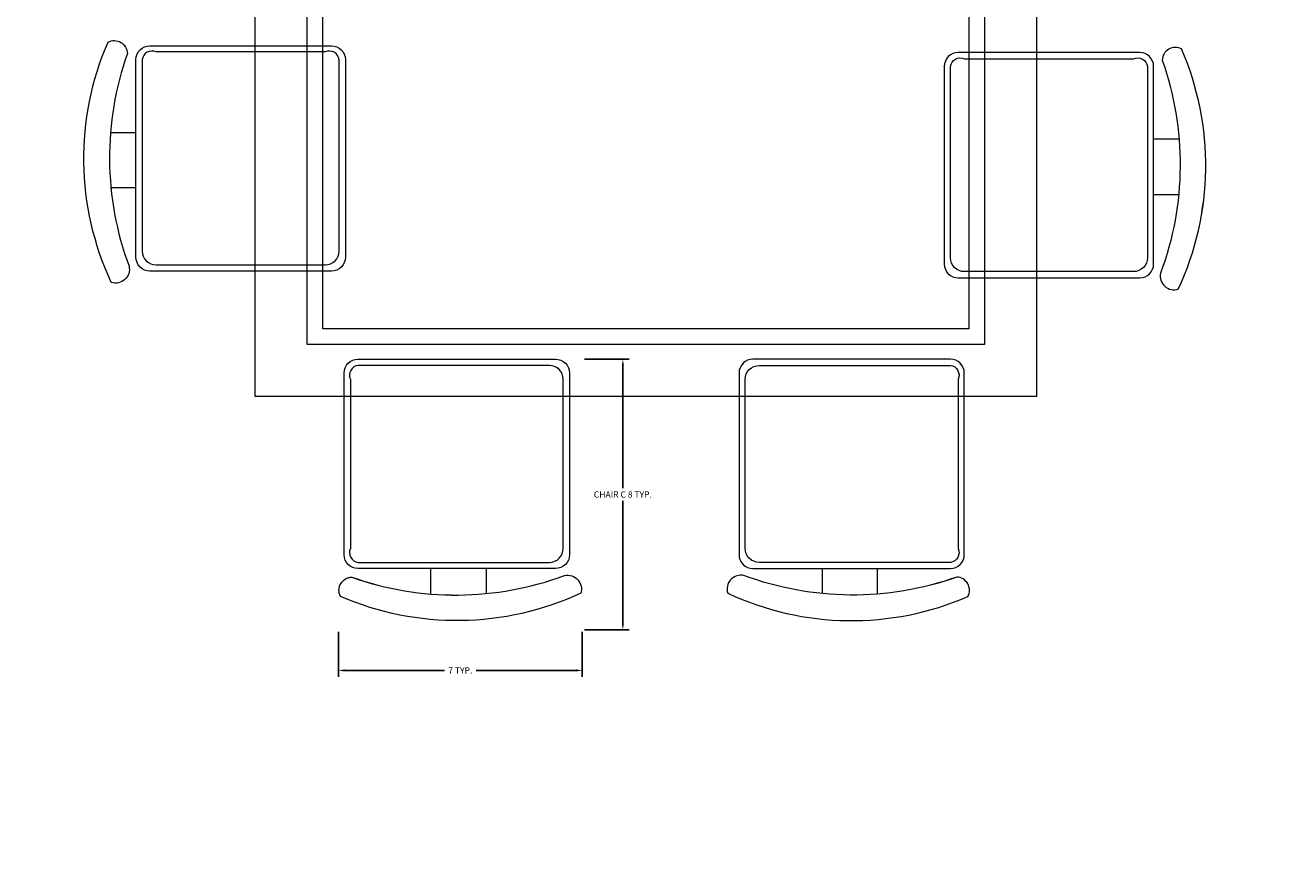
# Model space of a CAD drawing. Units: inches. Extents: x 1962 to 2771, y 1245 to 2660.
# Tile 87 of 114: x 2272 to 2308, y 2260 to 2284. Entities that reach past the tile are written whole.
import ezdxf

# ---------------------------------------------------------------- set-up
doc = ezdxf.new("R2010")
doc.units = ezdxf.units.IN
doc.layers.add('A-ANNO-DIMS', color=2, linetype='Continuous', lineweight=18)
doc.layers.add('A-FURN', color=8, linetype='Continuous', lineweight=13)
doc.styles.get("Standard").update_dxf_attribs({"font": 'arial.ttf'})
doc.dimstyles.get("Standard").update_dxf_attribs({"dimtxt": 0.18, "dimasz": 0.18, "dimexe": 0.18, "dimexo": 0.0625, "dimgap": 0.09, "dimtad": 0, "dimtih": 1, "dimtoh": 1, "dimdec": 4, "dimzin": 0, "dimdsep": 46, "dimtxsty": 'Standard', "dimcen": 0.09, "dimadec": 0, "dimazin": 0, "dimtfac": 1, "dimtdec": 4, "dimtofl": 0, "dimtmove": 0, "dimatfit": 3, "dimfxl": 1, "dimtolj": 1, "dimtzin": 0, "dimarcsym": 0})

# ---------------------------------------------------------------- blocks, each defined once
blk = doc.blocks.new('DINING-TABLE')
for points in [[(0, 13.512), (22.52, 13.512), (22.52, 0), (0, 0)], [(0, 13.512), (22.52, 13.512), (22.52, 0), (0, 0)], [(1.501, 12.011), (21.019, 12.011), (21.019, 1.502), (1.501, 1.502)], [(1.501, 12.011), (21.019, 12.011), (21.019, 1.501), (1.501, 1.501)], [(1.952, 11.561), (20.568, 11.561), (20.568, 1.952), (1.952, 1.952)], [(1.952, 11.56), (20.568, 11.56), (20.568, 1.952), (1.952, 1.952)]]:
    blk.add_lwpolyline(points, close=True)
blk = doc.blocks.new('DINING-CHAIR-C')
for points in [[(6.242, 1.501), (0.548, 1.501, -0.414214), (0.149, 1.899), (0.149, 7.135, -0.414214), (0.548, 7.534), (6.242, 7.534, -0.414214), (6.64, 7.135), (6.64, 1.899, -0.414214), (6.242, 1.501)], [(6.242, 1.501), (0.548, 1.501, -0.414214), (0.149, 1.899), (0.149, 7.135, -0.414214), (0.548, 7.533), (6.242, 7.533, -0.414214), (6.641, 7.135), (6.641, 1.899, -0.414214), (6.242, 1.501)], [(4.242, 1.501), (4.242, 0.781, 0.064759)], [(4.242, 1.501), (4.242, 0.78, 0.064759)], [(6.502, 1.301, -0.578392), (6.967, 0.79, -0.214524), (0.043, 0.697, -0.552014), (0.368, 1.255, 0.175809), (6.502, 1.301)], [(6.502, 1.301, -0.578392), (6.967, 0.79, -0.214524), (0.043, 0.697, -0.552014), (0.368, 1.254, 0.175809), (6.502, 1.301)]]:
    blk.add_lwpolyline(points, format="xyb")
for points in [[(0.55, 1.68), (6.063, 1.68, 0.414214), (6.461, 2.079), (6.461, 6.956, 0.414214), (6.063, 7.354), (0.55, 7.354, 0.512069), (0.329, 6.956), (0.329, 2.079, 0.512069)], [(0.55, 1.68), (6.063, 1.68, 0.414214), (6.461, 2.078), (6.461, 6.955, 0.414214), (6.063, 7.354), (0.55, 7.354, 0.512069), (0.329, 6.955), (0.329, 2.078, 0.512069)]]:
    blk.add_lwpolyline(points, format="xyb", close=True)
for points in [[(2.648, 0.768), (2.648, 1.501)], [(2.648, 0.767), (2.648, 1.501)]]:
    blk.add_lwpolyline(points)
blk = doc.blocks.new('*D38')
at = {"layer": 'A-ANNO-DIMS', "color": 0, "lineweight": -2, "transparency": 16777216}
for p, q in [((2288.118, 2274.618), (2289.405, 2274.618)), ((2289.225, 2274.438), (2289.225, 2270.903)), ((2289.225, 2267.001), (2289.225, 2270.537)), ((2288.118, 2266.821), (2289.405, 2266.821))]:
    blk.add_line(p, q, dxfattribs=at)
at = {"layer": 'A-ANNO-DIMS', "color": 0, "transparency": 16777216}
for points in [[(2289.195, 2274.438), (2289.255, 2274.438), (2289.225, 2274.618)], [(2289.195, 2267.001), (2289.255, 2267.001), (2289.225, 2266.821)]]:
    blk.add_solid(points, dxfattribs=at)
at = {"layer": 'Defpoints', "color": 0, "transparency": 16777216}
for p in [(2288.056, 2274.618), (2289.225, 2274.618), (2288.056, 2266.821)]:
    blk.add_point(p, dxfattribs=at)
at = {"layer": 'A-ANNO-DIMS', "color": 0, "transparency": 16777216, "insert": (2289.225, 2270.72), "char_height": 0.18, "attachment_point": 5}
blk.add_mtext('\\A1;CHAIR C 8 TYP.', dxfattribs=at)
blk = doc.blocks.new('*D39')
at = {"layer": 'A-ANNO-DIMS', "color": 0, "lineweight": -2, "transparency": 16777216}
for p, q in [((2281.028, 2266.759), (2281.028, 2265.471)), ((2288.056, 2266.759), (2288.056, 2265.471)), ((2281.208, 2265.651), (2284.084, 2265.651)), ((2287.876, 2265.651), (2284.999, 2265.651))]:
    blk.add_line(p, q, dxfattribs=at)
at = {"layer": 'A-ANNO-DIMS', "color": 0, "transparency": 16777216}
for points in [[(2281.208, 2265.681), (2281.208, 2265.621), (2281.028, 2265.651)], [(2287.876, 2265.681), (2287.876, 2265.621), (2288.056, 2265.651)]]:
    blk.add_solid(points, dxfattribs=at)
at = {"layer": 'Defpoints', "color": 0, "transparency": 16777216}
for p in [(2281.028, 2266.821), (2288.056, 2266.821), (2288.056, 2265.651)]:
    blk.add_point(p, dxfattribs=at)
at = {"layer": 'A-ANNO-DIMS', "color": 0, "transparency": 16777216, "insert": (2284.542, 2265.651), "char_height": 0.18, "attachment_point": 5}
blk.add_mtext('\\A1;7 TYP.', dxfattribs=at)
blk = doc.blocks.new('*D40')
at = {"layer": 'A-ANNO-DIMS', "color": 0, "lineweight": -2, "transparency": 16777216}
for p, q in [((2072.02, 2033.906), (2072.02, 2583.474)), ((2660.807, 2524.406), (2660.807, 2583.474)), ((2072.2, 2583.294), (2366.02, 2583.294)), ((2660.627, 2583.294), (2366.808, 2583.294))]:
    blk.add_line(p, q, dxfattribs=at)
at = {"layer": 'A-ANNO-DIMS', "color": 0, "transparency": 16777216}
for points in [[(2072.2, 2583.324), (2072.2, 2583.264), (2072.02, 2583.294)], [(2660.627, 2583.324), (2660.627, 2583.264), (2660.807, 2583.294)]]:
    blk.add_solid(points, dxfattribs=at)
at = {"layer": 'Defpoints', "color": 0, "transparency": 16777216}
for p in [(2660.807, 2583.294), (2660.807, 2524.344), (2072.02, 2033.844)]:
    blk.add_point(p, dxfattribs=at)
at = {"layer": 'A-ANNO-DIMS', "color": 0, "transparency": 16777216, "insert": (2366.414, 2583.294), "char_height": 0.18, "attachment_point": 5}
blk.add_mtext('\\A1;588.8', dxfattribs=at)

msp = doc.modelspace()

# ---------------------------------------------------------------- linework, layer by layer
at = {"layer": 'A-FURN'}
for points in [[(2274.9962, 2277.2945, -0.5783921), (2274.4852, 2276.8298, -0.2145244), (2274.3923, 2283.7537, -0.552014), (2274.9497, 2283.4284, 0.1758094), (2274.9962, 2277.2945)], [(2274.9962, 2277.2943, -0.5783921), (2274.4852, 2276.8296, -0.2145244), (2274.3923, 2283.7534, -0.552014), (2274.9497, 2283.4282, 0.1758094), (2274.9962, 2277.2943)], [(2275.1959, 2283.2492, -0.4142136), (2275.5943, 2283.6476), (2280.8302, 2283.6476, -0.4142136), (2281.2286, 2283.2492), (2281.2286, 2277.5548, -0.4142136), (2280.8302, 2277.1564), (2275.5943, 2277.1564, -0.4142136), (2275.1959, 2277.5548), (2275.1959, 2283.2492)], [(2275.1959, 2283.249, -0.4142136), (2275.5943, 2283.6474), (2280.8303, 2283.6474, -0.4142136), (2281.2286, 2283.249), (2281.2286, 2277.5545, -0.4142136), (2280.8303, 2277.1561), (2275.5943, 2277.1561, -0.4142136), (2275.1959, 2277.5545), (2275.1959, 2283.249)], [(2304.7659, 2283.2334, -0.1758092), (2304.7195, 2277.0995, 0.5783921), (2305.2304, 2276.6348, 0.2145244), (2305.3233, 2283.5587, 0.552014), (2304.7659, 2283.2334, -0.065079)], [(2304.7659, 2283.2331, -0.1758092), (2304.7195, 2277.0993, 0.5783921), (2305.2305, 2276.6346, 0.2145244), (2305.3234, 2283.5584, 0.552014), (2304.7659, 2283.2331, -0.065079)], [(2304.5197, 2283.0542, 0.4142136), (2304.1214, 2283.4526), (2298.8854, 2283.4526, 0.4142136), (2298.487, 2283.0542), (2298.487, 2277.3597, 0.4142136), (2298.8854, 2276.9614), (2304.1214, 2276.9614, 0.4142136), (2304.5197, 2277.3597), (2304.5197, 2283.0542)], [(2304.5198, 2283.054, 0.4142136), (2304.1214, 2283.4524), (2298.8854, 2283.4524, 0.4142136), (2298.487, 2283.054), (2298.487, 2277.3595, 0.4142136), (2298.8854, 2276.9611), (2304.1214, 2276.9611, 0.4142136), (2304.5198, 2277.3595), (2304.5198, 2283.054)], [(2275.1959, 2279.5549), (2274.4757, 2279.5549, 0.0647586)], [(2275.1959, 2279.5547), (2274.4757, 2279.5547, 0.0647586)], [(2304.5197, 2279.3599), (2305.2399, 2279.3599, -0.0647586)], [(2304.5198, 2279.3597), (2305.2399, 2279.3597, -0.0647586)], [(2298.6658, 2268.5856, 0.4142136), (2299.0642, 2268.984), (2299.0642, 2274.2199, 0.4142136), (2298.6658, 2274.6183), (2292.9714, 2274.6183, 0.4142136), (2292.573, 2274.2199), (2292.573, 2268.984, 0.4142136), (2292.9714, 2268.5856), (2298.6658, 2268.5856)], [(2298.6659, 2268.5854, 0.4142136), (2299.0642, 2268.9837), (2299.0642, 2274.2197, 0.4142136), (2298.6659, 2274.6181), (2292.9714, 2274.6181, 0.4142136), (2292.573, 2274.2197), (2292.573, 2268.9837, 0.4142136), (2292.9714, 2268.5854), (2298.6659, 2268.5854)], [(2298.845, 2268.3394, -0.1758093), (2292.7111, 2268.3859, 0.5783921), (2292.2464, 2267.8749, 0.2145244), (2299.1703, 2267.782, 0.552014), (2298.845, 2268.3394, -0.065079)], [(2298.845, 2268.3392, -0.1758093), (2292.7111, 2268.3856, 0.5783921), (2292.2465, 2267.8747, 0.2145244), (2299.1703, 2267.7818, 0.552014), (2298.845, 2268.3392, -0.065079)], [(2294.9716, 2268.5856), (2294.9716, 2267.8654, -0.0647586)], [(2294.9716, 2268.5854), (2294.9716, 2267.8652, -0.0647586)]]:
    msp.add_lwpolyline(points, format="xyb", dxfattribs=at)
for points in [[(2275.3754, 2283.2468), (2275.3754, 2277.7342, 0.4142136), (2275.7738, 2277.3359), (2280.6508, 2277.3359, 0.4142136), (2281.0492, 2277.7342), (2281.0492, 2283.2468, 0.5120695), (2280.6508, 2283.4681), (2275.7738, 2283.4681, 0.5120695)], [(2275.3754, 2283.2466), (2275.3754, 2277.734, 0.4142136), (2275.7738, 2277.3356), (2280.6508, 2277.3356, 0.4142136), (2281.0492, 2277.734), (2281.0492, 2283.2466, 0.5120695), (2280.6508, 2283.4679), (2275.7738, 2283.4679, 0.5120695)], [(2304.3403, 2283.0518), (2304.3403, 2277.5392, -0.4142136), (2303.9419, 2277.1408), (2299.0649, 2277.1408, -0.4142136), (2298.6665, 2277.5392), (2298.6665, 2283.0518, -0.5120695), (2299.0649, 2283.2731), (2303.9419, 2283.2731, -0.5120695)], [(2304.3403, 2283.0516), (2304.3403, 2277.539, -0.4142136), (2303.9419, 2277.1406), (2299.0649, 2277.1406, -0.4142136), (2298.6665, 2277.539), (2298.6665, 2283.0516, -0.5120695), (2299.0649, 2283.2729), (2303.9419, 2283.2729, -0.5120695)], [(2298.6634, 2268.7651), (2293.1508, 2268.7651, -0.4142136), (2292.7525, 2269.1635), (2292.7525, 2274.0405, -0.4142136), (2293.1508, 2274.4388), (2298.6634, 2274.4388, -0.5120695), (2298.8848, 2274.0405), (2298.8848, 2269.1635, -0.5120695)], [(2298.6634, 2268.7648), (2293.1509, 2268.7648, -0.4142136), (2292.7525, 2269.1632), (2292.7525, 2274.0402, -0.4142136), (2293.1509, 2274.4386), (2298.6634, 2274.4386, -0.5120695), (2298.8848, 2274.0402), (2298.8848, 2269.1632, -0.5120695)]]:
    msp.add_lwpolyline(points, format="xyb", close=True, dxfattribs=at)
for points in [[(2274.4626, 2281.1489), (2275.1959, 2281.1489)], [(2274.4626, 2281.1487), (2275.1959, 2281.1487)], [(2305.253, 2280.9539), (2304.5197, 2280.9539)], [(2305.253, 2280.9537), (2304.5198, 2280.9537)], [(2296.5655, 2267.8523), (2296.5655, 2268.5856)], [(2296.5655, 2267.8521), (2296.5655, 2268.5854)]]:
    msp.add_lwpolyline(points, dxfattribs=at)

# ---------------------------------------------------------------- block references
for name, p in [('DINING-TABLE', (2278.6278, 2273.5392)), ('DINING-CHAIR-C', (2281.0449, 2267.0848))]:
    msp.add_blockref(name, p, dxfattribs=at)

# ---------------------------------------------------------------- dimensions: what is measured, and where the dimension line sits
at = {"layer": 'A-ANNO-DIMS'}
dim = msp.add_linear_dim(base=(2660.8074, 2583.2937), p1=(2072.0204, 2033.8437), p2=(2660.8074, 2524.3437), dimstyle='Standard', override={"dimdec": 1, "dimlfac": 1, "dimrnd": 0, "dimzin": 0, "dimdsep": 46, "dimlunit": 2}, dxfattribs=at)
dim.commit()
dim.dimension.update_dxf_attribs({"geometry": '*D40', "text_midpoint": (2366.4139, 2583.2937)})
dim = msp.add_linear_dim(base=(2289.2251, 2274.6183), p1=(2288.0555, 2266.8211), p2=(2288.0555, 2274.6183), angle=90, text='CHAIR C <> TYP.', dimstyle='Standard', override={"dimdec": 0, "dimlfac": 1, "dimrnd": 0, "dimzin": 0, "dimdsep": 46, "dimlunit": 2}, dxfattribs=at)
dim.commit()
dim.dimension.update_dxf_attribs({"geometry": '*D38', "text_midpoint": (2289.2251, 2270.7197)})
dim = msp.add_linear_dim(base=(2288.0555, 2265.6515), p1=(2281.0275, 2266.8211), p2=(2288.0555, 2266.8211), text='<> TYP.', dimstyle='Standard', override={"dimdec": 0, "dimlfac": 1, "dimrnd": 0, "dimzin": 0, "dimdsep": 46, "dimlunit": 2}, dxfattribs=at)
dim.commit()
dim.dimension.update_dxf_attribs({"geometry": '*D39', "text_midpoint": (2284.5415, 2265.6515)})

doc.saveas('drawing.dxf')
